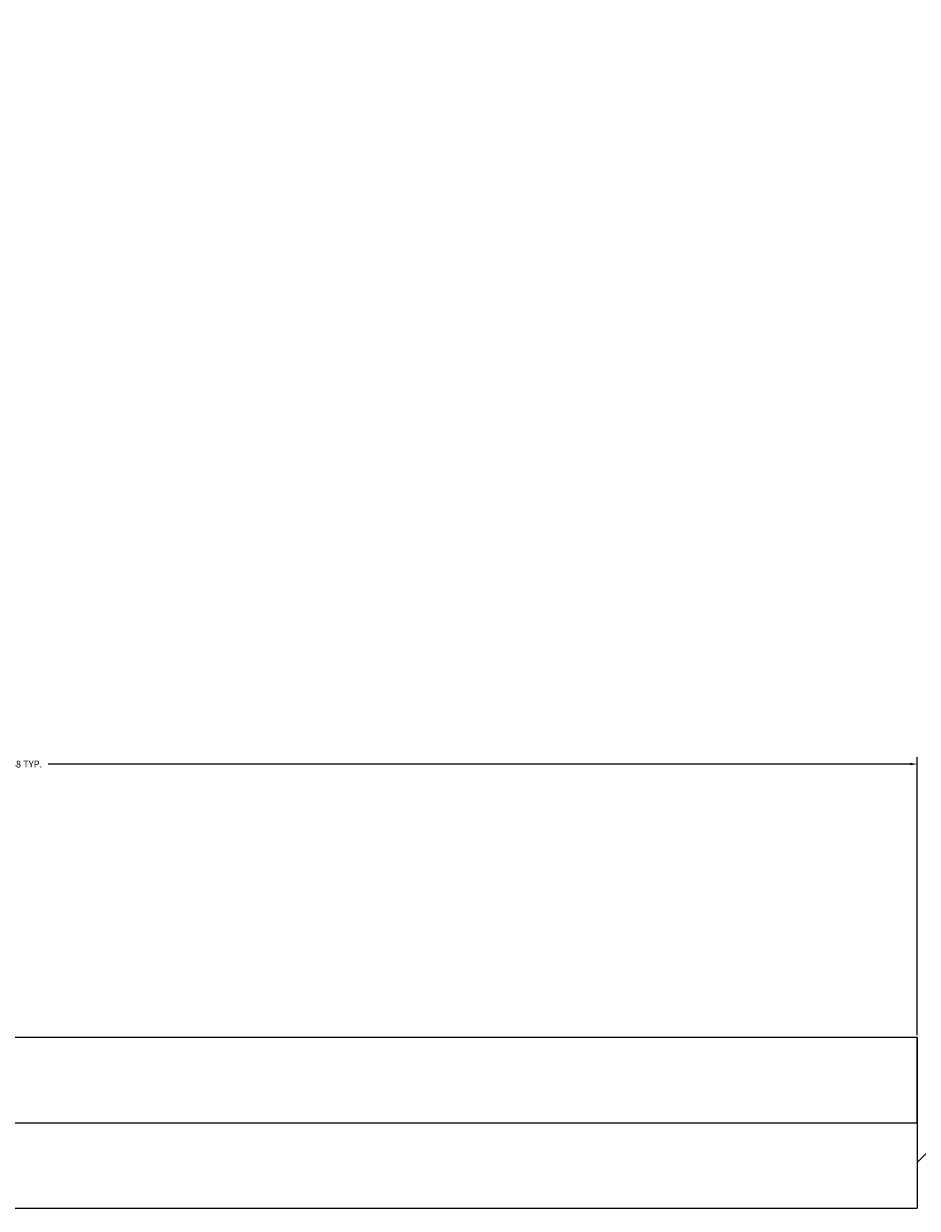
# Model space of a CAD drawing. Units: inches. Extents: x 1885 to 2748, y 783 to 2421.
# Tile 47 of 117: x 2263 to 2287, y 1558 to 1589. Entities that reach past the tile are written whole.
import ezdxf

# ---------------------------------------------------------------- set-up
doc = ezdxf.new("R2010")
doc.units = ezdxf.units.IN
doc.layers.add('A-ANNO-DIMS', color=2, linetype='Continuous', lineweight=18)
doc.layers.add('A-GLAZ', color=181, linetype='Continuous', lineweight=18)
doc.layers.add('A-WALL-PATT', color=85, linetype='Continuous', lineweight=13, true_color=0x58ba48)
doc.styles.get("Standard").update_dxf_attribs({"font": 'arial.ttf'})
doc.dimstyles.get("Standard").update_dxf_attribs({"dimtxt": 0.18, "dimasz": 0.18, "dimexe": 0.18, "dimexo": 0.0625, "dimgap": 0.09, "dimtad": 0, "dimtih": 1, "dimtoh": 1, "dimdec": 4, "dimzin": 0, "dimdsep": 46, "dimtxsty": 'Standard', "dimcen": 0.09, "dimadec": 0, "dimazin": 0, "dimtfac": 1, "dimtdec": 4, "dimtofl": 0, "dimtmove": 0, "dimatfit": 3, "dimfxl": 1, "dimtolj": 1, "dimtzin": 0, "dimarcsym": 0})

# ---------------------------------------------------------------- blocks, each defined once
blk = doc.blocks.new('WIN-48')
for p, q in [((48.003, 4.496), (0.003, 4.496)), ((48.003, 2.246), (48.003, 4.496)), ((48.003, 4.496), (48.003, -0.004)), ((0.003, 2.246), (48.003, 2.246)), ((0.003, -0.004), (48.003, -0.004))]:
    blk.add_line(p, q)
blk = doc.blocks.new('*D25')
at = {"layer": 'A-ANNO-DIMS', "color": 0, "lineweight": -2, "transparency": 16777216}
for p, q in [((2238.613, 1562.568), (2238.613, 1569.886)), ((2286.613, 1562.568), (2286.613, 1569.886)), ((2238.793, 1569.706), (2261.495, 1569.706)), ((2286.433, 1569.706), (2263.732, 1569.706))]:
    blk.add_line(p, q, dxfattribs=at)
at = {"layer": 'A-ANNO-DIMS', "color": 0, "transparency": 16777216}
for points in [[(2238.793, 1569.736), (2238.793, 1569.676), (2238.613, 1569.706)], [(2286.433, 1569.736), (2286.433, 1569.676), (2286.613, 1569.706)]]:
    blk.add_solid(points, dxfattribs=at)
at = {"layer": 'Defpoints', "color": 0, "transparency": 16777216}
for p in [(2286.613, 1569.706), (2238.613, 1562.506), (2286.613, 1562.506)]:
    blk.add_point(p, dxfattribs=at)
at = {"layer": 'A-ANNO-DIMS', "color": 0, "transparency": 16777216, "insert": (2262.613, 1569.706), "char_height": 0.18, "attachment_point": 5}
blk.add_mtext('\\A1;WINDOW 48 TYP.', dxfattribs=at)

msp = doc.modelspace()

# ---------------------------------------------------------------- hatches: boundary and pattern name
at = {"layer": 'A-WALL-PATT'}
h = msp.add_hatch(dxfattribs=at)
h.set_pattern_fill('ANSI32', color=256)
h.paths.add_polyline_path([(2007.772, 2318.006), (1980.774, 2318.006), (1980.774, 2281.215), (1985.274, 2281.215), (1985.274, 2313.506), (2007.772, 2313.506), (2007.772, 2315.756)])
h.paths.add_polyline_path([(2094.324, 2318.006), (2067.772, 2318.006), (2067.772, 2313.506), (2094.324, 2313.506), (2094.324, 2315.756)])
h.paths.add_polyline_path([(2131.367, 2315.756), (2131.367, 2318.006), (2131.189, 2318.006), (2112.609, 2318.006), (2112.609, 2313.506), (2117.274, 2313.506), (2117.274, 2255.201), (2121.774, 2255.201), (2121.774, 2313.506), (2131.367, 2313.506)])
h.paths.add_polyline_path([(2190.512, 2318.006), (2155.367, 2318.006), (2155.367, 2313.506), (2169.774, 2313.506), (2169.774, 2229.506), (2121.774, 2229.506), (2121.774, 2233.451), (2119.524, 2233.451), (2117.274, 2233.451), (2117.274, 2201.101), (2121.774, 2201.101), (2121.774, 2225.006), (2169.774, 2225.006), (2169.774, 2165.006), (2306.274, 2165.006), (2306.274, 2066.006), (2310.774, 2066.006), (2344.274, 2066.006), (2486.274, 2066.006), (2486.274, 1886.006), (2483.02, 1886.006), (2483.02, 1881.506), (2486.274, 1881.506), (2486.274, 1880.678), (2490.774, 1880.678), (2490.774, 2070.506), (2344.274, 2070.506), (2310.774, 2070.506), (2310.774, 2165.006), (2310.774, 2173.636), (2308.524, 2173.636), (2306.274, 2173.636), (2306.274, 2169.506), (2174.274, 2169.506), (2174.274, 2313.506), (2190.512, 2313.506), (2190.512, 2315.756)])
h.paths.add_polyline_path([(1985.274, 2221.215), (1980.774, 2221.215), (1980.774, 2165.006), (1992.774, 2165.006), (1992.774, 2141.927), (1997.274, 2141.927), (1997.274, 2165.006), (2117.274, 2165.006), (2117.274, 2163.126), (2121.774, 2163.126), (2121.774, 2172.734), (2119.524, 2172.734), (2117.274, 2172.734), (2117.274, 2169.506), (1985.274, 2169.506)])
h.paths.add_polyline_path([(1997.274, 2105.927), (1992.774, 2105.927), (1992.774, 2070.506), (2016.774, 2070.506), (2016.774, 2059.123), (2019.024, 2059.123), (2021.274, 2059.123), (2021.274, 2070.506), (2117.274, 2070.506), (2117.274, 2022.506), (2114.423, 2022.506), (2114.423, 2018.006), (2123.627, 2018.006), (2123.627, 2020.256), (2123.627, 2022.506), (2121.774, 2022.506), (2121.774, 2142.587), (2119.524, 2142.587), (2117.274, 2142.587), (2117.274, 2075.006), (1997.274, 2075.006)])
h.paths.add_polyline_path([(2092.029, 2020.256), (2092.029, 2022.506), (2021.274, 2022.506), (2021.274, 2035.123), (2016.774, 2035.123), (2016.774, 2018.006), (2016.774, 1978.784), (2021.274, 1978.784), (2021.274, 2018.006), (2092.029, 2018.006)])
h.paths.add_polyline_path([(2260.938, 2022.506), (2153.105, 2022.506), (2153.105, 2020.256), (2153.105, 2018.006), (2155.274, 2018.006), (2155.274, 1886.006), (2107.629, 1886.006), (2107.629, 1881.506), (2182.911, 1881.506), (2182.911, 1883.756), (2182.911, 1886.006), (2159.774, 1886.006), (2159.774, 2018.006), (2260.938, 2018.006), (2260.938, 2020.256)])
h.paths.add_polyline_path([(2047.629, 1883.756), (2047.629, 1886.006), (2021.274, 1886.006), (2021.274, 1918.784), (2019.024, 1918.784), (2016.774, 1918.784), (2016.774, 1881.506), (2047.629, 1881.506)])
h.paths.add_polyline_path([(2306.361, 1883.756), (2306.361, 1886.006), (2296.274, 1886.006), (2296.274, 1982.006), (2316.535, 1982.006), (2316.535, 1984.256), (2316.535, 1986.506), (2296.274, 1986.506), (2296.274, 2022.506), (2289.276, 2022.506), (2289.276, 2018.006), (2291.774, 2018.006), (2291.774, 1886.006), (2242.911, 1886.006), (2242.911, 1881.506), (2306.361, 1881.506)], flags=17)
h.paths.add_polyline_path([(1985.274, 1843.006), (2021.6, 1843.006), (2021.534, 1845.441), (2021.477, 1847.506), (1980.774, 1847.506), (1980.774, 1809.446), (1985.274, 1809.446)])
h.paths.add_polyline_path([(2131.482, 1845.256), (2131.482, 1847.506), (2081.534, 1847.506), (2081.534, 1843.006), (2117.274, 1843.006), (2117.274, 1784.147), (2119.524, 1784.147), (2121.774, 1784.147), (2121.774, 1843.006), (2131.482, 1843.006)])
h.paths.add_polyline_path([(2203.886, 1847.506), (2155.482, 1847.506), (2155.482, 1843.006), (2169.774, 1843.006), (2169.774, 1759.006), (2121.774, 1759.006), (2121.774, 1761.457), (2117.274, 1761.457), (2117.274, 1730.429), (2121.774, 1730.429), (2121.774, 1754.506), (2177.421, 1754.506), (2177.421, 1756.756), (2177.421, 1759.006), (2174.274, 1759.006), (2174.274, 1843.006), (2203.886, 1843.006)])
h.paths.add_polyline_path([(2335.554, 1845.256), (2335.554, 1847.506), (2239.886, 1847.506), (2239.886, 1843.006), (2306.274, 1843.006), (2306.274, 1759.006), (2199.486, 1759.006), (2199.486, 1754.506), (2310.774, 1754.506), (2310.774, 1843.006), (2335.554, 1843.006)])
h.paths.add_polyline_path([(2348.774, 2022.506), (2344.274, 2022.506), (2344.274, 1986.506), (2341.681, 1986.506), (2341.681, 1982.006), (2344.274, 1982.006), (2344.274, 1886.006), (2330.361, 1886.006), (2330.361, 1881.506), (2361.627, 1881.506), (2361.627, 1883.756), (2361.627, 1886.006), (2348.774, 1886.006)], flags=17)
h.paths.add_polyline_path([(2283.251, 2315.756), (2283.251, 2318.006), (2238.512, 2318.006), (2238.512, 2313.506), (2283.251, 2313.506)], flags=17)
h.paths.add_polyline_path([(2363.274, 2348.006), (2388.677, 2348.006), (2388.677, 2350.256), (2388.677, 2352.506), (2358.774, 2352.506), (2358.774, 2348.006), (2358.774, 2318.006), (2344.481, 2318.006), (2344.481, 2313.506), (2358.774, 2313.506), (2358.774, 2229.506), (2310.774, 2229.506), (2310.774, 2231.952), (2306.274, 2231.952), (2306.274, 2205.611), (2310.774, 2205.611), (2310.774, 2225.006), (2358.774, 2225.006), (2358.774, 2211.506), (2452.329, 2211.506), (2452.329, 2213.756), (2452.329, 2216.006), (2363.274, 2216.006), (2363.274, 2318.006)])
h.paths.add_polyline_path([(2310.774, 2313.506), (2320.481, 2313.506), (2320.481, 2315.756), (2320.481, 2318.006), (2302.728, 2318.006), (2302.728, 2313.506), (2306.274, 2313.506), (2306.274, 2251.076), (2310.774, 2251.076)], flags=17)
h.paths.add_polyline_path([(2490.774, 2352.506), (2486.274, 2352.506), (2448.677, 2352.506), (2448.677, 2348.006), (2486.274, 2348.006), (2486.274, 2318.006), (2486.274, 2216.006), (2481.78, 2216.006), (2481.78, 2211.506), (2486.274, 2211.506), (2486.274, 2165.006), (2493.289, 2165.006), (2493.289, 2167.256), (2493.289, 2169.506), (2490.774, 2169.506), (2490.774, 2313.506), (2494.429, 2313.506), (2494.429, 2318.006), (2490.774, 2318.006)])
h.paths.add_polyline_path([(2534.653, 2318.006), (2515.691, 2318.006), (2515.691, 2313.506), (2534.653, 2313.506), (2534.653, 2315.756)])
h.paths.add_polyline_path([(2618.274, 2318.006), (2594.653, 2318.006), (2594.653, 2313.506), (2613.774, 2313.506), (2613.774, 2281.706), (2618.274, 2281.706)])
h.paths.add_polyline_path([(2618.274, 2221.706), (2613.774, 2221.706), (2613.774, 2169.506), (2554.019, 2169.506), (2554.019, 2165.006), (2613.774, 2165.006), (2613.774, 2152.878), (2618.274, 2152.878)])
h.paths.add_polyline_path([(2618.274, 2128.878), (2616.024, 2128.878), (2613.774, 2128.878), (2613.774, 2117.006), (2529.774, 2117.006), (2529.774, 2165.006), (2532.848, 2165.006), (2532.848, 2169.506), (2522.867, 2169.506), (2522.867, 2165.006), (2525.274, 2165.006), (2525.274, 2117.006), (2525.274, 2112.506), (2525.274, 2108.576), (2529.774, 2108.576), (2529.774, 2112.506), (2613.774, 2112.506), (2613.774, 2080.19), (2618.274, 2080.19)])
h.paths.add_polyline_path([(2618.274, 2044.19), (2616.024, 2044.19), (2613.774, 2044.19), (2613.774, 2015.506), (2529.774, 2015.506), (2529.774, 2088.582), (2527.524, 2088.582), (2525.274, 2088.582), (2525.274, 2011.006), (2613.774, 2011.006), (2613.774, 1956.755), (2618.274, 1956.755)])
h.paths.add_polyline_path([(2618.274, 1881.506), (2618.274, 1896.755), (2613.774, 1896.755), (2613.774, 1881.506), (2613.774, 1847.506), (2592.715, 1847.506), (2592.715, 1843.006), (2613.774, 1843.006), (2613.774, 1765.006), (2613.774, 1760.506), (2609.621, 1760.506), (2609.621, 1756.006), (2613.774, 1756.006), (2613.774, 1660.006), (2608.544, 1660.006), (2608.544, 1655.506), (2613.774, 1655.506), (2613.774, 1508.158), (2618.274, 1508.158)])
h.paths.add_polyline_path([(2565.774, 1843.006), (2568.997, 1843.006), (2568.997, 1847.506), (2490.774, 1847.506), (2490.774, 1849.7), (2488.524, 1849.7), (2486.274, 1849.7), (2486.274, 1847.506), (2477.274, 1847.506), (2477.274, 1838.506), (2477.274, 1821.493), (2486.274, 1821.493), (2486.274, 1838.506), (2561.274, 1838.506), (2561.274, 1765.006), (2486.274, 1765.006), (2486.274, 1786.157), (2477.274, 1786.157), (2477.274, 1765.006), (2477.274, 1756.006), (2486.274, 1756.006), (2565.774, 1756.006), (2585.621, 1756.006), (2585.621, 1758.256), (2585.621, 1760.506), (2565.774, 1760.506), (2565.774, 1765.006)])
h.paths.add_polyline_path([(2486.274, 1651.006), (2561.274, 1651.006), (2561.274, 1567.006), (2486.274, 1567.006), (2486.274, 1591.321), (2477.274, 1591.321), (2477.274, 1567.006), (2477.274, 1558.006), (2477.274, 1555.439), (2481.774, 1555.439), (2481.774, 1558.006), (2568.653, 1558.006), (2568.653, 1560.256), (2568.653, 1562.506), (2565.774, 1562.506), (2565.774, 1655.506), (2584.544, 1655.506), (2584.544, 1657.756), (2584.544, 1660.006), (2565.774, 1660.006), (2486.274, 1660.006), (2477.274, 1660.006), (2477.274, 1651.006), (2477.274, 1632.989), (2486.274, 1632.989)])
h.paths.add_polyline_path([(2449.967, 1883.756), (2449.967, 1886.006), (2421.627, 1886.006), (2421.627, 1881.506), (2449.967, 1881.506)], flags=17)
h.paths.add_polyline_path([(2447.274, 1847.506), (2395.554, 1847.506), (2395.554, 1843.006), (2442.774, 1843.006), (2442.774, 1809.27), (2447.274, 1809.27)])
h.paths.add_polyline_path([(1985.274, 1749.446), (1980.774, 1749.446), (1980.774, 1694.504), (1985.274, 1694.504), (1985.274, 1694.506), (1986.897, 1694.506), (1986.897, 1697.78), (1986.897, 1699.006), (1985.274, 1699.006)])
h.paths.add_polyline_path([(2152.774, 1699.006), (2121.774, 1699.006), (2121.774, 1703.668), (2119.524, 1703.668), (2117.274, 1703.668), (2117.274, 1699.006), (2009.219, 1699.006), (2009.219, 1694.506), (2148.274, 1694.506), (2148.274, 1692.631), (2152.774, 1692.631)])
h.paths.add_polyline_path([(2016.274, 1694.506), (2011.774, 1694.506), (2011.774, 1558.006), (2040.806, 1558.006), (2040.806, 1560.256), (2040.806, 1562.506), (2016.274, 1562.506)])
h.paths.add_polyline_path([(2152.774, 1663.017), (2150.524, 1663.017), (2148.274, 1663.017), (2148.274, 1562.506), (2100.806, 1562.506), (2100.806, 1558.006), (2165.119, 1558.006), (2165.119, 1560.256), (2165.119, 1562.506), (2152.774, 1562.506), (2152.774, 1610.506), (2224.774, 1610.506), (2224.774, 1607.99), (2229.274, 1607.99), (2229.274, 1615.006), (2152.774, 1615.006)])
h.paths.add_polyline_path([(2238.613, 1560.256), (2238.613, 1562.506), (2229.274, 1562.506), (2229.274, 1588.756), (2227.024, 1588.763), (2224.774, 1588.771), (2224.774, 1562.506), (2189.119, 1562.506), (2189.119, 1558.006), (2238.613, 1558.006)])
h.paths.add_polyline_path([(2336.024, 1560.256), (2336.024, 1562.506), (2310.774, 1562.506), (2310.774, 1656.347), (2308.524, 1656.347), (2306.274, 1656.347), (2306.274, 1562.506), (2286.613, 1562.506), (2286.613, 1558.006), (2336.024, 1558.006)])
h.paths.add_polyline_path([(2447.274, 1690.968), (2445.024, 1690.968), (2442.774, 1690.968), (2442.774, 1687.006), (2306.274, 1687.006), (2306.274, 1680.75), (2310.774, 1680.75), (2310.774, 1682.506), (2442.774, 1682.506), (2442.774, 1562.506), (2396.024, 1562.506), (2396.024, 1558.006), (2447.274, 1558.006)])
h.paths.add_polyline_path([(2447.274, 1749.27), (2445.024, 1749.27), (2442.774, 1749.27), (2442.774, 1717.232), (2447.274, 1717.232)])
h.paths.add_polyline_path([(2044.674, 1521.756), (2044.674, 1524.006), (2007.274, 1524.006), (2007.274, 1503.49), (2009.524, 1503.49), (2011.774, 1503.49), (2011.774, 1519.506), (2044.674, 1519.506)])
h.paths.add_polyline_path([(2177.969, 1521.756), (2177.969, 1524.006), (2104.674, 1524.006), (2104.674, 1519.506), (2145.774, 1519.506), (2145.774, 1387.506), (2143.37, 1387.506), (2143.37, 1383.006), (2251.585, 1383.006), (2251.585, 1385.256), (2251.585, 1387.506), (2150.274, 1387.506), (2150.274, 1519.506), (2177.969, 1519.506)])
h.paths.add_polyline_path([(2298.704, 1524.006), (2237.969, 1524.006), (2237.969, 1519.506), (2282.274, 1519.506), (2282.274, 1387.506), (2279.683, 1387.506), (2279.683, 1383.006), (2286.774, 1383.006), (2286.774, 1419.006), (2312.451, 1419.006), (2312.451, 1421.256), (2312.451, 1423.506), (2286.774, 1423.506), (2286.774, 1519.506), (2298.704, 1519.506), (2298.704, 1521.722)], flags=17)
h.paths.add_polyline_path([(2361.897, 1521.756), (2361.897, 1524.006), (2322.704, 1524.006), (2322.704, 1519.506), (2334.774, 1519.506), (2334.774, 1423.506), (2331.93, 1423.506), (2331.93, 1419.006), (2334.774, 1419.006), (2334.774, 1387.506), (2334.774, 1383.228), (2339.274, 1383.228), (2339.274, 1387.506), (2339.274, 1519.506), (2361.897, 1519.506)], flags=17)
h.paths.add_polyline_path([(2447.274, 1521.756), (2447.274, 1524.006), (2421.897, 1524.006), (2421.897, 1519.506), (2447.274, 1519.506)], flags=17)
h.paths.add_polyline_path([(2481.774, 1529.6), (2479.524, 1529.6), (2477.274, 1529.6), (2477.274, 1524.006), (2474.489, 1524.006), (2474.489, 1519.506), (2477.274, 1519.506), (2477.274, 1334.506), (2296.774, 1334.506), (2296.774, 1240.506), (2160.274, 1240.506), (2160.274, 1180.506), (2112.274, 1180.506), (2112.274, 1207.692), (2110.024, 1207.692), (2107.774, 1207.692), (2107.774, 1171.609), (2112.274, 1171.609), (2112.274, 1176.006), (2160.274, 1176.006), (2160.274, 1092.006), (2144.221, 1092.006), (2144.221, 1087.506), (2189.497, 1087.506), (2189.497, 1089.756), (2189.497, 1092.006), (2164.774, 1092.006), (2164.774, 1236.006), (2296.774, 1236.006), (2296.774, 1231.912), (2301.274, 1231.912), (2301.274, 1330.006), (2481.774, 1330.006), (2481.774, 1387.506)])
h.paths.add_polyline_path([(2618.274, 1448.158), (2613.774, 1448.158), (2613.774, 1382.506), (2529.774, 1382.506), (2525.274, 1382.506), (2525.274, 1307.062), (2529.774, 1307.062), (2529.774, 1378.006), (2613.774, 1378.006), (2613.774, 1354.988), (2618.274, 1354.988)])
h.paths.add_polyline_path([(2618.274, 1318.988), (2613.774, 1318.988), (2613.774, 1281.006), (2529.774, 1281.006), (2529.774, 1283.786), (2527.524, 1283.786), (2525.274, 1283.786), (2525.274, 1228.506), (2516.794, 1228.506), (2516.794, 1224.006), (2533.484, 1224.006), (2533.484, 1226.256), (2533.484, 1228.506), (2529.774, 1228.506), (2529.774, 1276.506), (2613.774, 1276.506), (2613.774, 1266.02), (2618.274, 1266.02)])
h.paths.add_polyline_path([(2618.274, 1134.964), (2613.774, 1134.964), (2613.774, 1092.006), (2594.545, 1092.006), (2594.545, 1087.506), (2618.274, 1087.506)])
h.paths.add_polyline_path([(2534.545, 1092.006), (2509.765, 1092.006), (2509.765, 1087.506), (2534.545, 1087.506), (2534.545, 1089.756)])
h.paths.add_polyline_path([(2481.274, 1224.006), (2484.117, 1224.006), (2484.117, 1226.256), (2484.117, 1228.506), (2476.774, 1228.506), (2476.774, 1198.506), (2471.61, 1198.506), (2471.61, 1194.006), (2476.774, 1194.006), (2476.774, 1062.006), (2436.894, 1062.006), (2436.894, 1057.506), (2476.774, 1057.506), (2481.274, 1057.506), (2481.274, 1062.006), (2481.274, 1087.506), (2485.354, 1087.506), (2485.354, 1089.756), (2485.354, 1092.006), (2481.274, 1092.006), (2481.274, 1117.506)])
h.paths.add_polyline_path([(2439.898, 1198.506), (2349.274, 1198.506), (2349.274, 1194.006), (2349.274, 1180.506), (2301.274, 1180.506), (2301.274, 1201.896), (2299.024, 1201.896), (2296.774, 1201.896), (2296.774, 1172.335), (2299.024, 1172.335), (2301.274, 1172.335), (2301.274, 1176.006), (2349.274, 1176.006), (2349.274, 1092.006), (2334.452, 1092.006), (2334.452, 1087.506), (2349.274, 1087.506), (2349.274, 1057.506), (2353.774, 1057.506), (2376.894, 1057.506), (2376.894, 1059.756), (2376.894, 1062.006), (2353.774, 1062.006), (2353.774, 1087.506), (2353.774, 1180.506), (2353.774, 1194.006), (2439.898, 1194.006), (2439.898, 1196.256)])
h.paths.add_polyline_path([(2270.596, 1089.756), (2270.596, 1092.006), (2249.497, 1092.006), (2249.497, 1087.506), (2270.596, 1087.506)], flags=17)
h.paths.add_polyline_path([(2310.452, 1092.006), (2301.274, 1092.006), (2301.274, 1153.292), (2296.774, 1153.292), (2296.774, 1092.006), (2293.786, 1092.006), (2293.786, 1087.506), (2310.452, 1087.506), (2310.452, 1089.756)], flags=17)
h.paths.add_polyline_path([(2112.274, 1150.328), (2110.024, 1150.328), (2107.774, 1150.328), (2107.774, 1092.006), (2104.465, 1092.006), (2104.465, 1087.506), (2120.221, 1087.506), (2120.221, 1089.756), (2120.221, 1092.006), (2112.274, 1092.006)])
h.paths.add_polyline_path([(2082.172, 1092.006), (2058.144, 1092.006), (2058.144, 1087.506), (2082.172, 1087.506), (2082.172, 1089.756)])
h.paths.add_polyline_path([(1975.774, 1145.638), (1971.274, 1145.638), (1971.274, 1087.506), (1980.774, 1087.506), (1998.144, 1087.506), (1998.144, 1089.756), (1998.144, 1092.006), (1985.274, 1092.006), (1975.774, 1092.006)])
h.paths.add_polyline_path([(2112.274, 1244.385), (2110.024, 1244.385), (2107.774, 1244.385), (2107.774, 1240.506), (1992.274, 1240.506), (1992.274, 1271.008), (1987.774, 1271.008), (1987.774, 1240.506), (1980.774, 1240.506), (1975.774, 1240.506), (1971.274, 1240.506), (1971.274, 1205.638), (1975.774, 1205.638), (1975.774, 1236.006), (2107.774, 1236.006), (2107.774, 1233.444), (2112.274, 1233.444), (2112.274, 1236.006)])
h.paths.add_polyline_path([(2112.274, 1383.006), (2114.783, 1383.006), (2114.783, 1385.256), (2114.783, 1387.506), (2102.476, 1387.506), (2102.476, 1383.006), (2107.774, 1383.006), (2107.774, 1335.006), (2011.774, 1335.006), (2011.774, 1349.939), (2007.274, 1349.939), (2007.274, 1335.006), (1987.774, 1335.006), (1987.774, 1330.506), (1987.774, 1307.008), (1992.274, 1307.008), (1992.274, 1330.506), (2007.274, 1330.506), (2107.774, 1330.506), (2107.774, 1264.711), (2112.274, 1264.711)])
h.paths.add_polyline_path([(2077.857, 1387.506), (2011.774, 1387.506), (2011.774, 1390.036), (2009.524, 1390.036), (2007.274, 1390.036), (2007.274, 1373.939), (2011.774, 1373.939), (2011.774, 1383.006), (2077.857, 1383.006)])
h.paths.add_polyline_path([(2011.774, 1443.49), (2007.274, 1443.49), (2007.274, 1410.248), (2011.774, 1410.248)])

# ---------------------------------------------------------------- block references
at = {"layer": 'A-GLAZ'}
msp.add_blockref('WIN-48', (2238.61, 1558.01), dxfattribs=at)

# ---------------------------------------------------------------- dimensions: what is measured, and where the dimension line sits
at = {"layer": 'A-ANNO-DIMS'}
dim = msp.add_linear_dim(base=(2286.613, 1569.706), p1=(2238.613, 1562.506), p2=(2286.613, 1562.506), text='WINDOW <> TYP.', dimstyle='Standard', override={"dimdec": 0, "dimlfac": 1, "dimrnd": 0, "dimzin": 0, "dimdsep": 46, "dimlunit": 2}, dxfattribs=at)
dim.commit()
dim.dimension.update_dxf_attribs({"geometry": '*D25', "text_midpoint": (2262.613, 1569.706)})

doc.saveas('drawing.dxf')
